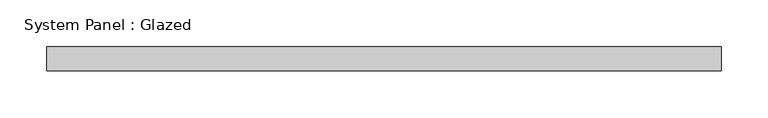
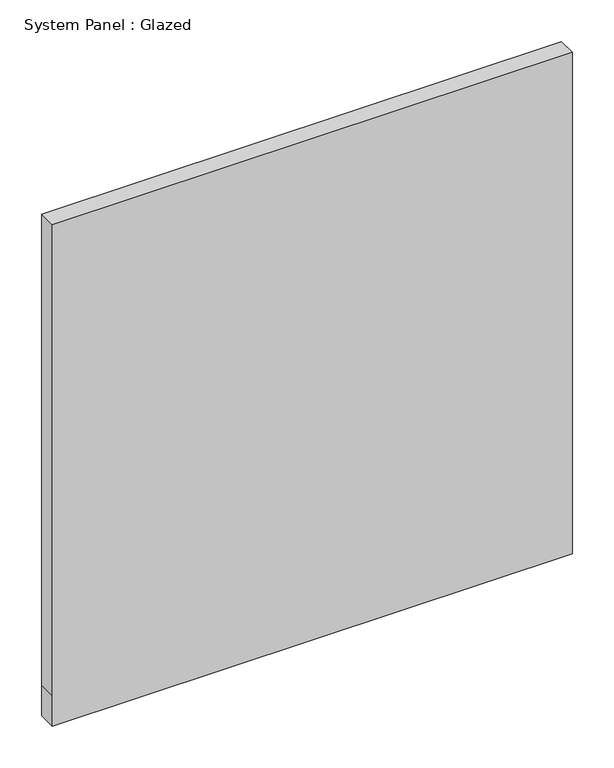
"""IFC4 building model written with IfcOpenShell, lengths in millimetres: plate geometry, System Panel : Glazed."""

from ifc_helpers import new_model, si_unit, frame, origin, place, context, project, spatial, polyline, outline, extrude, source, transform, mapped, element, save


def system_panel_glazed_72d2109d(model_context):
    return source(origin(), model_context, "Body", "SweptSolid", [
        extrude(outline(polyline([(0.0, -358.775), (0.0, 358.775), (44.45, 358.775), (731.566916, 358.775), (731.566916, -358.775), (44.45, -358.775), (0.0, -358.775)])), frame((0.0, 19.05, 0.0), z_axis=(0.0, 1.0, 0.0), x_axis=(0.0, 0.0, 1.0)), (0.0, 0.0, 1.0), 25.4),
    ])


if __name__ == "__main__":
    model = new_model("IFC4")
    model_context = context("Model", 3, world=origin())
    ifc_project = project(units=[si_unit("LENGTHUNIT", "METRE", prefix="MILLI")], contexts=[model_context])
    site = spatial("IfcSite", under=ifc_project)
    building = spatial("IfcBuilding", under=site)
    placement = place(None, origin())
    system_panel_glazed_shape = system_panel_glazed_72d2109d(model_context)
    element("IfcPlate", 1, ObjectType="System Panel : Glazed", at=placement, inside=building, context=model_context, shape_type="MappedRepresentation", body=[
        mapped(system_panel_glazed_shape, transform((0.0, 0.0, 0.0), x_axis=(1.0, 0.0, 0.0), y_axis=(0.0, 1.0, 0.0), z_axis=(0.0, 0.0, 1.0))),
    ])
    save(model, "model.ifc")

# Revit data of these elements
# Type "System Panel : Glazed"
#   Construction Type Id = "GSP4R"
#   Analytic Construction = "1/8 in Pilkington single glazing"
#   Visual Light Transmittance = 0.9
#   Solar Heat Gain Coefficient = 0.86
#   Heat Transfer Coefficient (U) = 1.18115 BTU/(h·ft²·°F)
#   Define Thermal Properties by = 1
# Element 1 (IfcPlate, "System Panel : Glazed")
#   Materials on its faces: "Glass"
# Materials
#   "Glass": class "Glass", colour RGB 0 128 192, transparency 0.75, Description = "Soda Lime Glass", Cost = 0
